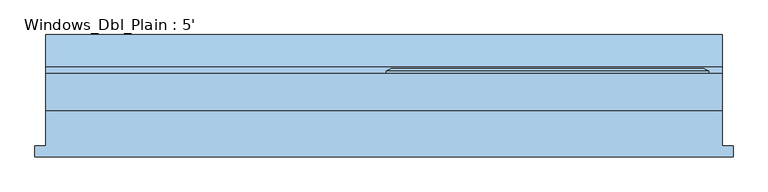
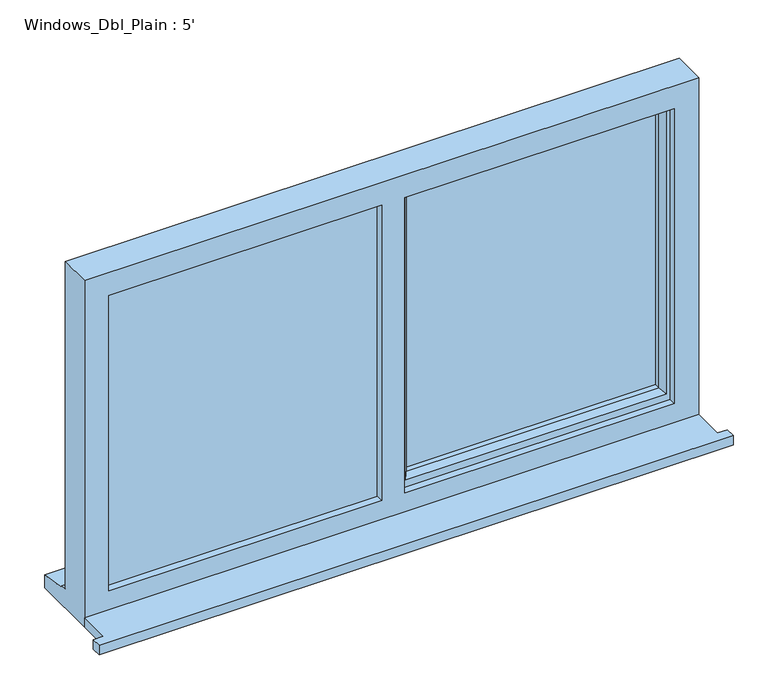
"""IFC4 building model written with IfcOpenShell, lengths in millimetres: window geometry, Windows_Dbl_Plain : 5'."""

from ifc_helpers import new_model, si_unit, frame, origin, place, context, project, spatial, polyline, outline, extrude, faceted_brep, source, transform, mapped, element, save


def windows_dbl_plain_5_907a13a5(model_context):
    return source(origin(), model_context, "Body", "SolidModel", [
        extrude(outline(polyline([(-1072.0, -123.2234322), (-1072.0, -98.2234322), (-1047.0, -98.2234322), (-1047.0, -17.8634322), (477.0, -17.8634322), (477.0, -98.2234322), (502.0, -98.2234322), (502.0, -123.2234322), (-1072.0, -123.2234322)])), frame((0.0, 0.0, 1200.0), z_axis=(0.0, 0.0, 1.0), x_axis=(1.0, 0.0, 0.0)), (0.0, 0.0, 1.0), 25.0),
        faceted_brep([(-280.0, 65.1365678, 2080.0), (-280.0, 70.9100705, 2080.0), (-280.0, 70.9100705, 1253.0), (-280.0, 65.1365678, 1253.0), (-270.0, 0.1365678, 2070.0), (-270.0, 65.1365678, 2070.0), (-270.0, 65.1365678, 1263.0), (-270.0, 0.1365678, 1263.0), (-230.0, 14.6294677, 2030.0), (-240.1480377, 0.1365678, 2040.1480377), (-240.1480377, 0.1365678, 1292.8519623), (-230.0, 14.6294677, 1303.0), (-230.0, 29.1365678, 2030.0), (-230.0, 29.1365678, 1303.0), (-240.0, 53.1365678, 2040.0), (-240.0, 29.1365678, 2040.0), (-240.0, 29.1365678, 1293.0), (-240.0, 53.1365678, 1293.0), (-230.0, 70.9100705, 2030.0), (-230.0, 53.1365678, 2030.0), (-230.0, 53.1365678, 1303.0), (-230.0, 70.9100705, 1303.0), (-247.4457548, 76.6835732, 2047.4457548), (-247.4457548, 76.6835732, 1285.5542452), (-269.2153903, 76.6835732, 2069.2153903), (-269.2153903, 76.6835732, 1263.7846097), (447.0, 70.9100705, 1253.0), (447.0, 65.1365678, 1253.0), (437.0, 65.1365678, 1263.0), (437.0, 0.1365678, 1263.0), (407.1480377, 0.1365678, 1292.8519623), (397.0, 14.6294677, 1303.0), (397.0, 29.1365678, 1303.0), (407.0, 29.1365678, 1293.0), (407.0, 53.1365678, 1293.0), (397.0, 53.1365678, 1303.0), (397.0, 70.9100705, 1303.0), (414.4457548, 76.6835732, 1285.5542452), (436.2153903, 76.6835732, 1263.7846097), (447.0, 70.9100705, 2080.0), (447.0, 65.1365678, 2080.0), (437.0, 65.1365678, 2070.0), (437.0, 0.1365678, 2070.0), (407.1480377, 0.1365678, 2040.1480377), (397.0, 14.6294677, 2030.0), (397.0, 29.1365678, 2030.0), (407.0, 29.1365678, 2040.0), (407.0, 53.1365678, 2040.0), (397.0, 53.1365678, 2030.0), (397.0, 70.9100705, 2030.0), (414.4457548, 76.6835732, 2047.4457548), (436.2153903, 76.6835732, 2069.2153903)], [[[0, 1, 2, 3]], [[4, 5, 6, 7]], [[8, 9, 10, 11]], [[12, 8, 11, 13]], [[14, 15, 16, 17]], [[18, 19, 20, 21]], [[22, 18, 21, 23]], [[1, 24, 25, 2]], [[3, 2, 26, 27]], [[7, 6, 28, 29]], [[11, 10, 30, 31]], [[13, 11, 31, 32]], [[17, 16, 33, 34]], [[21, 20, 35, 36]], [[23, 21, 36, 37]], [[2, 25, 38, 26]], [[27, 26, 39, 40]], [[29, 28, 41, 42]], [[31, 30, 43, 44]], [[32, 31, 44, 45]], [[34, 33, 46, 47]], [[36, 35, 48, 49]], [[37, 36, 49, 50]], [[26, 38, 51, 39]], [[40, 39, 1, 0]], [[3, 27, 40, 0], [5, 41, 28, 6]], [[42, 41, 5, 4]], [[7, 29, 42, 4], [9, 43, 30, 10]], [[44, 43, 9, 8]], [[45, 44, 8, 12]], [[15, 46, 33, 16], [13, 32, 45, 12]], [[47, 46, 15, 14]], [[17, 34, 47, 14], [19, 48, 35, 20]], [[49, 48, 19, 18]], [[50, 49, 18, 22]], [[24, 51, 38, 25], [23, 37, 50, 22]], [[39, 51, 24, 1]]]),
        extrude(outline(polyline([(2050.0, -310.0), (2070.0, -310.0), (2070.0, -1007.0), (1263.0, -1007.0), (1263.0, -310.0), (1283.0, -310.0), (1283.0, -987.0), (2050.0, -987.0), (2050.0, -310.0)])), frame((0.0, 24.1365678, 0.0), z_axis=(0.0, 1.0, 0.0), x_axis=(0.0, 0.0, 1.0)), (0.0, 0.0, 1.0), 41.0),
        faceted_brep([(477.0, -17.8634322, 2110.0), (-1047.0, -17.8634322, 2110.0), (-1047.0, -17.8634322, 1200.0), (477.0, -17.8634322, 1200.0), (417.0, -17.8634322, 2050.0), (417.0, -17.8634322, 1275.0), (-252.0, -17.8634322, 1275.0), (-252.0, -17.8634322, 2050.0), (-310.0, -17.8634322, 2050.0), (-310.0, -17.8634322, 1275.0), (-987.0, -17.8634322, 1275.0), (-987.0, -17.8634322, 2050.0), (-1047.0, 65.1365678, 2110.0), (-1047.0, 65.1365678, 1251.0), (-1047.0, 80.1365678, 1249.68767), (-1047.0, 80.1365678, 1244.7449676), (-1047.0, 152.6365678, 1233.8088847), (-1047.0, 152.6365678, 1200.0), (477.0, 65.1365678, 2110.0), (477.0, 65.1365678, 1251.0), (-1007.0, 65.1365678, 2070.0), (-1007.0, 65.1365678, 1263.0), (-310.0, 65.1365678, 1263.0), (-310.0, 65.1365678, 2070.0), (-270.0, 65.1365678, 2070.0), (-270.0, 65.1365678, 1263.0), (437.0, 65.1365678, 1263.0), (437.0, 65.1365678, 2070.0), (-1007.0, 0.1365678, 2070.0), (-1007.0, 0.1365678, 1263.0), (-300.0, 0.1365678, 2070.0), (-300.0, 0.1365678, 1263.0), (-310.0, 0.1365678, 2050.0), (-987.0, 0.1365678, 2050.0), (-987.0, 0.1365678, 1275.0), (-310.0, 0.1365678, 1275.0), (-270.0, 0.1365678, 2070.0), (437.0, 0.1365678, 2070.0), (437.0, 0.1365678, 1263.0), (-270.0, 0.1365678, 1263.0), (417.0, 0.1365678, 2050.0), (-252.0, 0.1365678, 2050.0), (-252.0, 0.1365678, 1275.0), (417.0, 0.1365678, 1275.0), (-310.0, 24.1365678, 2070.0), (-300.0, 24.1365678, 2070.0), (477.0, 152.6365678, 1200.0), (477.0, 152.6365678, 1233.8088847), (477.0, 80.1365678, 1244.7449676), (477.0, 80.1365678, 1249.68767), (-300.0, 24.1365678, 1263.0), (-310.0, 24.1365678, 1263.0)], [[[0, 1, 2, 3], [4, 5, 6, 7], [8, 9, 10, 11]], [[2, 1, 12, 13, 14, 15, 16, 17]], [[13, 12, 18, 19], [20, 21, 22, 23], [24, 25, 26, 27]], [[21, 20, 28, 29]], [[28, 30, 31, 29], [32, 33, 34, 35]], [[36, 37, 38, 39], [40, 41, 42, 43]], [[33, 11, 10, 34]], [[1, 0, 18, 12]], [[28, 20, 23, 44, 45, 30]], [[27, 37, 36, 24]], [[11, 33, 32, 8]], [[40, 4, 7, 41]], [[19, 18, 0, 3, 46, 47, 48, 49]], [[27, 26, 38, 37]], [[4, 40, 43, 5]], [[45, 50, 31, 30]], [[50, 45, 44, 51]], [[51, 44, 23, 22]], [[25, 24, 36, 39]], [[41, 7, 6, 42]], [[8, 32, 35, 9]], [[46, 3, 2, 17]], [[47, 46, 17, 16]], [[48, 47, 16, 15]], [[49, 48, 15, 14]], [[19, 49, 14, 13]], [[22, 21, 29, 31, 50, 51]], [[26, 25, 39, 38]], [[6, 5, 43, 42]], [[35, 34, 10, 9]]]),
        extrude(outline(polyline([(-1007.0, 24.1365678), (-300.0, 24.1365678), (-300.0, 0.1365678), (-1007.0, 0.1365678), (-1007.0, 24.1365678)])), frame((0.0, 0.0, 1263.0), z_axis=(0.0, 0.0, 1.0), x_axis=(1.0, 0.0, 0.0)), (0.0, 0.0, 1.0), 807.0),
        extrude(outline(polyline([(407.0, 29.1365678), (-240.0, 29.1365678), (-240.0, 53.1365678), (407.0, 53.1365678), (407.0, 29.1365678)])), frame((0.0, 0.0, 1293.0), z_axis=(0.0, 0.0, 1.0), x_axis=(1.0, 0.0, 0.0)), (0.0, 0.0, 1.0), 747.0),
    ])


if __name__ == "__main__":
    model = new_model("IFC4")
    model_context = context("Model", 3, world=origin())
    ifc_project = project(units=[si_unit("LENGTHUNIT", "METRE", prefix="MILLI")], contexts=[model_context])
    site = spatial("IfcSite", under=ifc_project)
    building = spatial("IfcBuilding", under=site)
    placement = place(None, origin())
    windows_dbl_plain_5_shape = windows_dbl_plain_5_907a13a5(model_context)
    element("IfcWindow", 1, ObjectType="Windows_Dbl_Plain : 5'", at=placement, inside=building, context=model_context, shape_type="MappedRepresentation", body=[
        mapped(windows_dbl_plain_5_shape, transform((0.0, 0.0, 0.0), x_axis=(1.0, 0.0, 0.0), y_axis=(0.0, 1.0, 0.0), z_axis=(0.0, 0.0, 1.0))),
    ])
    save(model, "model.ifc")

# Revit data of these elements
# Type "Windows_Dbl_Plain : 5'"
#   Type Mark = "58"
#   Operation = "DoublePanelVertical"
#   Construction Type Id = "GSP4R"
#   Manufacturer = "Revit"
#   Keynote = "L10"
#   Analytic Construction = "1/8 in Pilkington single glazing"
#   Wrap Layers (Ext) from Ext = 0.336286 ft
#   Wrap Layers (Int) from Ext = 0.582349 ft
#   Window Board Projection = 0.082021 ft
#   Window Board Extension = 0.082021 ft
#   Visual Light Transmittance = 0.9
#   Solar Heat Gain Coefficient = 0.78
#   Rough Width = 5.0 ft
#   Rough Height = 2.985564 ft
#   Height = 2.985564 ft
#   Width = 5.0 ft
#   Heat Transfer Coefficient (U) = 3.6886 W/(m²·K)
#   Glazing Thickness = 0.07874 ft
#   FrameOffset - External = 0.164042 ft
#   Frame Depth = 0.213255 ft
#   Default Head Height = 6.922572 ft
#   Cill Depth = 0.287073 ft
#   Cavity Closer Width = 0.164042 ft
#   Cavity Closer Offset from Ext = 0.336286 ft
#   Cavity Closer Depth = 0.278871 ft
#   Vis - Cavity Closers = yes
#   Define Thermal Properties by = 1
#   Material Trim = Window Frame
#   Material Glass = Glass
#   Material Frame = Window Frame
#   Wall Closure = (empty or 0)
# Element 1 (IfcWindow, "Windows_Dbl_Plain : 5'")
#   Materials on its faces: "Window Frame", "Glass"
# Materials
#   "Window Frame": colour RGB 249 249 249, transparency 0, Keynote = "L10", Cost = 0
#   "Glass": class "Glass", colour RGB 0 128 192, transparency 0.9, Description = "Soda Lime Glass", Cost = 0
